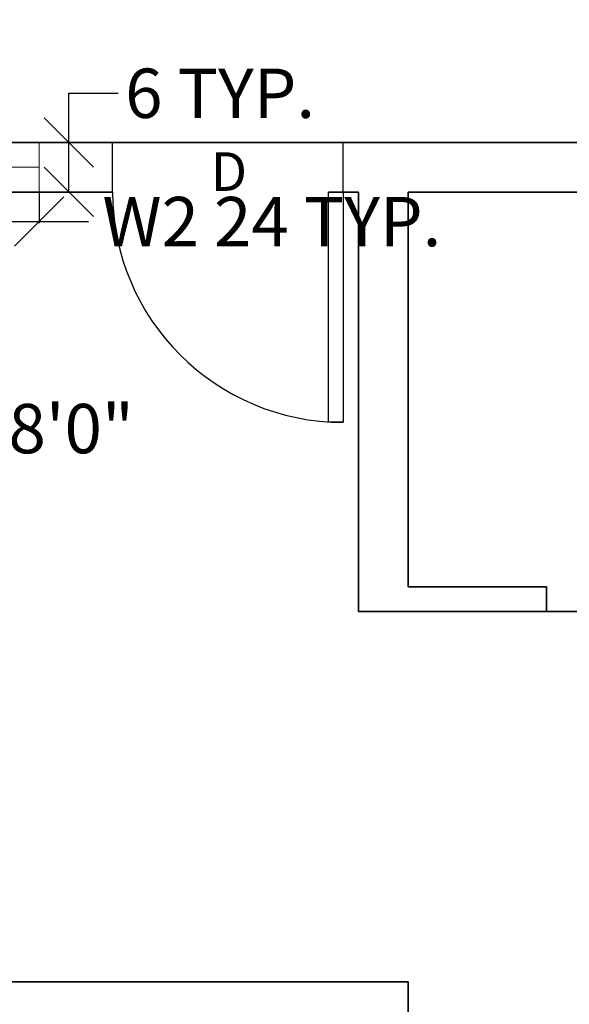
# Model space of a CAD drawing. Units: inches. Extents: x -1198 to -69, y -512 to 437.
# Tile 17 of 50: x -934 to -867, y 158 to 278. Entities that reach past the tile are written whole.
import ezdxf

# ---------------------------------------------------------------- set-up
doc = ezdxf.new("R2010")
doc.units = ezdxf.units.IN
doc.header["$MEASUREMENT"] = 0
for name, color, linetype, lineweight in [('A-ANNO-DIMS', 2, 'Continuous', 18), ('A-ANNO-SYMB', 7, 'Continuous', 18), ('A-AREA-IDEN', 7, 'Continuous', 18), ('A-WALL', 7, 'Continuous', 35), ('Doors', 140, 'Continuous', 25), ('windows', 160, 'Continuous', 18)]:
    doc.layers.add(name, color=color, linetype=linetype, lineweight=lineweight)
doc.styles.get("Standard").update_dxf_attribs({"font": 'arial.ttf'})
doc.dimstyles.get("Standard").update_dxf_attribs({"dimtxt": 6, "dimasz": 6, "dimexe": 0.18, "dimexo": 0.0625, "dimgap": 0.09, "dimtad": 0, "dimtih": 1, "dimtoh": 1, "dimdec": 0, "dimzin": 0, "dimdsep": 46, "dimlunit": 4, "dimtxsty": 'Standard', "dimblk": 'OBLIQUE', "dimcen": 0.09, "dimadec": 0, "dimazin": 0, "dimtfac": 1, "dimtdec": 0, "dimtofl": 0, "dimtmove": 0, "dimatfit": 3, "dimfxl": 1, "dimtolj": 1, "dimtzin": 0, "dimarcsym": 0})

# ---------------------------------------------------------------- blocks, each defined once
blk = doc.blocks.new('*U4')
for p, q in [((0, 0), (0, -6)), ((28, 0), (28, -6))]:
    blk.add_line(p, q)
blk.add_lwpolyline([(0, 0), (0, 28), (1.75, 28), (1.75, 0)], close=True)
blk.add_arc((0, 0), 28, 0, 90)
blk = doc.blocks.new('WIN-W2-24')
at = {"ltscale": 10}
for p, q in [((0, 6), (0, 0)), ((24, 6), (24, 0)), ((0, 3), (24, 3))]:
    blk.add_line(p, q, dxfattribs=at)
blk = doc.blocks.new('_Oblique')
at = {"color": 0, "linetype": 'ByBlock', "lineweight": -2}
blk.add_line((-0.5, -0.5), (0.5, 0.5), dxfattribs=at)
blk = doc.blocks.new('*D48')
at = {"layer": 'A-ANNO-DIMS', "color": 0, "lineweight": -2, "ltscale": 10, "transparency": 16777216}
for p, q in [((-955.56, 257.17), (-955.56, 253.45)), ((-931.56, 257.17), (-931.56, 253.45)), ((-955.56, 253.63), (-931.56, 253.63)), ((-931.56, 253.63), (-925.56, 253.63))]:
    blk.add_line(p, q, dxfattribs=at)
at = {"layer": 'DEFPOINTS', "color": 0, "ltscale": 10, "transparency": 16777216}
for p in [(-955.56, 257.23), (-931.56, 257.23), (-931.56, 253.63)]:
    blk.add_point(p, dxfattribs=at)
at = {"layer": 'A-ANNO-DIMS', "color": 0, "lineweight": -2, "ltscale": 10, "transparency": 16777216, "xscale": 6, "yscale": 6, "zscale": 6, "rotation": 180}
blk.add_blockref('_Oblique', (-955.56, 253.63), dxfattribs=at)
at = {"layer": 'A-ANNO-DIMS', "color": 0, "lineweight": -2, "ltscale": 10, "transparency": 16777216, "xscale": 6, "yscale": 6, "zscale": 6}
blk.add_blockref('_Oblique', (-931.56, 253.63), dxfattribs=at)
at = {"layer": 'A-ANNO-DIMS', "color": 0, "ltscale": 10, "transparency": 16777216, "insert": (-903.29, 253.63), "char_height": 6, "attachment_point": 5}
blk.add_mtext('\\A1;W2 24 TYP.', dxfattribs=at)
blk = doc.blocks.new('*D49')
at = {"layer": 'A-ANNO-DIMS', "color": 0, "lineweight": -2, "ltscale": 10, "transparency": 16777216}
for p, q in [((-927.96, 263.23), (-927.96, 269.23)), ((-927.96, 269.23), (-921.96, 269.23)), ((-931.5, 263.23), (-927.78, 263.23)), ((-927.96, 257.23), (-927.96, 263.23)), ((-931.5, 257.23), (-927.78, 257.23))]:
    blk.add_line(p, q, dxfattribs=at)
at = {"layer": 'DEFPOINTS', "color": 0, "ltscale": 10, "transparency": 16777216}
for p in [(-931.56, 263.23), (-927.96, 263.23), (-931.56, 257.23)]:
    blk.add_point(p, dxfattribs=at)
at = {"layer": 'A-ANNO-DIMS', "color": 0, "lineweight": -2, "ltscale": 10, "transparency": 16777216, "xscale": 6, "yscale": 6, "zscale": 6}
for p, rotation in [((-927.96, 263.23), 90), ((-927.96, 257.23), 270)]:
    blk.add_blockref('_Oblique', p, dxfattribs=dict(at, rotation=rotation))
at = {"layer": 'A-ANNO-DIMS', "color": 0, "ltscale": 10, "transparency": 16777216, "insert": (-909.58, 269.23), "char_height": 6, "attachment_point": 5}
blk.add_mtext('\\A1;6 TYP.', dxfattribs=at)

msp = doc.modelspace()

# ---------------------------------------------------------------- linework, layer by layer
at = {"layer": 'A-WALL', "ltscale": 10}
for p, q in [((-697.7509, 263.2277), (-1018.7509, 263.2277)), ((-1012.7509, 257.2277), (-922.6458, 257.2277)), ((-896.3958, 257.2277), (-892.7509, 257.2277)), ((-892.7509, 257.2277), (-892.7509, 206.2277)), ((-886.7509, 257.2277), (-886.7509, 209.2277)), ((-811.7509, 257.2277), (-886.7509, 257.2277)), ((-869.9135, 209.2277), (-886.7509, 209.2277)), ((-869.9135, 209.2277), (-869.9135, 206.2277)), ((-811.7509, 206.2277), (-892.7509, 206.2277)), ((-886.7509, 161.2277), (-1012.7509, 161.2277)), ((-886.7509, 161.2277), (-886.7509, 35.2277))]:
    msp.add_line(p, q, dxfattribs=at)

# ---------------------------------------------------------------- block references
at = {"layer": 'Doors', "rotation": 180}
msp.add_blockref('*U4', (-894.6458, 257.2277), dxfattribs=at)
at = {"layer": 'windows'}
msp.add_blockref('WIN-W2-24', (-955.559, 257.228), dxfattribs=at)

# ---------------------------------------------------------------- texts
at = {"layer": 'A-ANNO-SYMB', "ltscale": 10}
msp.add_text('D', height=4.6996, dxfattribs=at).set_placement((-910.7131, 257.3605))
at = {"layer": 'A-AREA-IDEN', "ltscale": 10, "insert": (-962.8292, 231.4637), "char_height": 6, "attachment_point": 1}
msp.add_mtext_dynamic_manual_height_columns('10\'0" x 8\'0"', width=57.976527, gutter_width=30, heights=[0], dxfattribs=at)

# ---------------------------------------------------------------- dimensions: what is measured, and where the dimension line sits
at = {"layer": 'A-ANNO-DIMS', "ltscale": 10}
dim = msp.add_linear_dim(base=(-927.9591, 263.2277), p1=(-931.5591, 257.2277), p2=(-931.5591, 263.2277), angle=90, text='<> TYP.', dimstyle='Standard', override={"dimdec": 0, "dimlfac": 1, "dimrnd": 0, "dimzin": 0, "dimdsep": 46, "dimlunit": 2}, dxfattribs=at)
dim.commit()
dim.dimension.update_dxf_attribs({"geometry": '*D49', "text_midpoint": (-909.5806, 269.2277)})
dim = msp.add_linear_dim(base=(-931.5591, 253.6277), p1=(-955.5591, 257.2277), p2=(-931.5591, 257.2277), text='W2 <> TYP.', dimstyle='Standard', override={"dimdec": 0, "dimlfac": 1, "dimrnd": 0, "dimzin": 0, "dimdsep": 46, "dimlunit": 2}, dxfattribs=at)
dim.commit()
dim.dimension.update_dxf_attribs({"geometry": '*D48', "text_midpoint": (-903.2925, 253.6277)})

doc.saveas('drawing.dxf')
